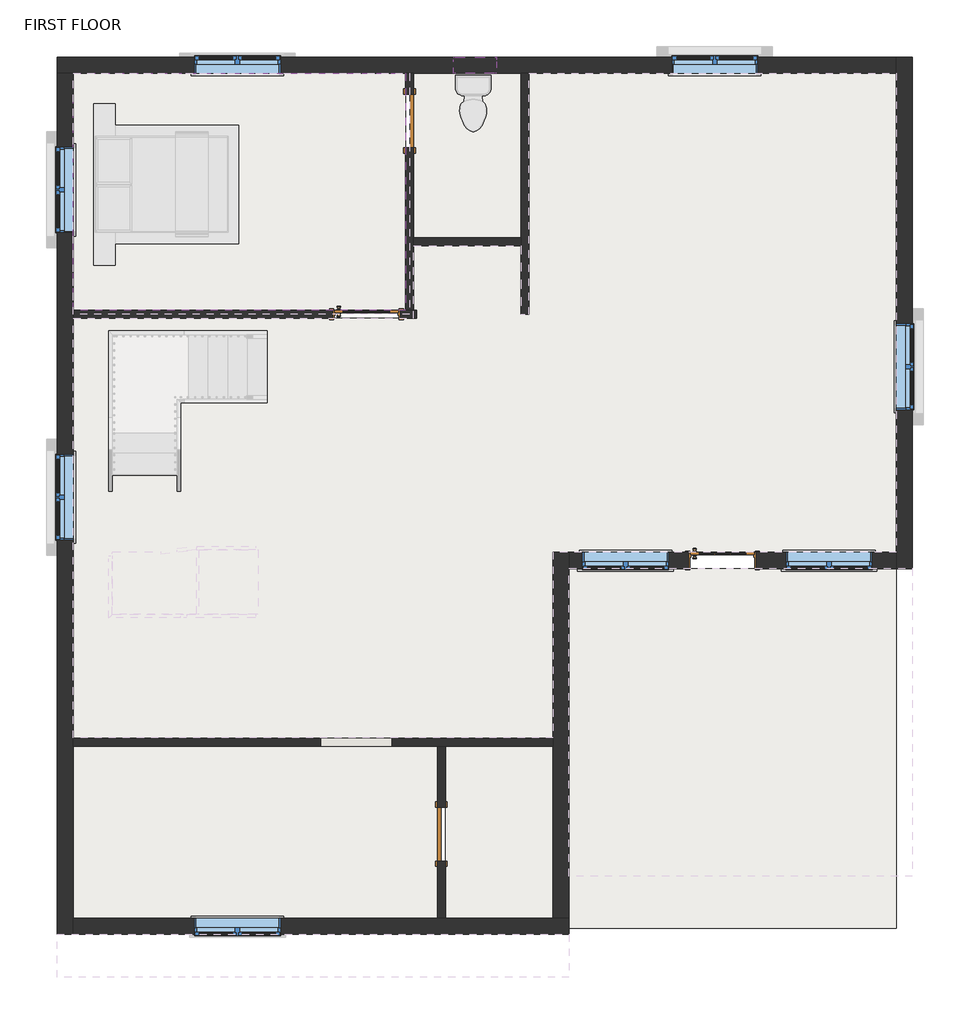
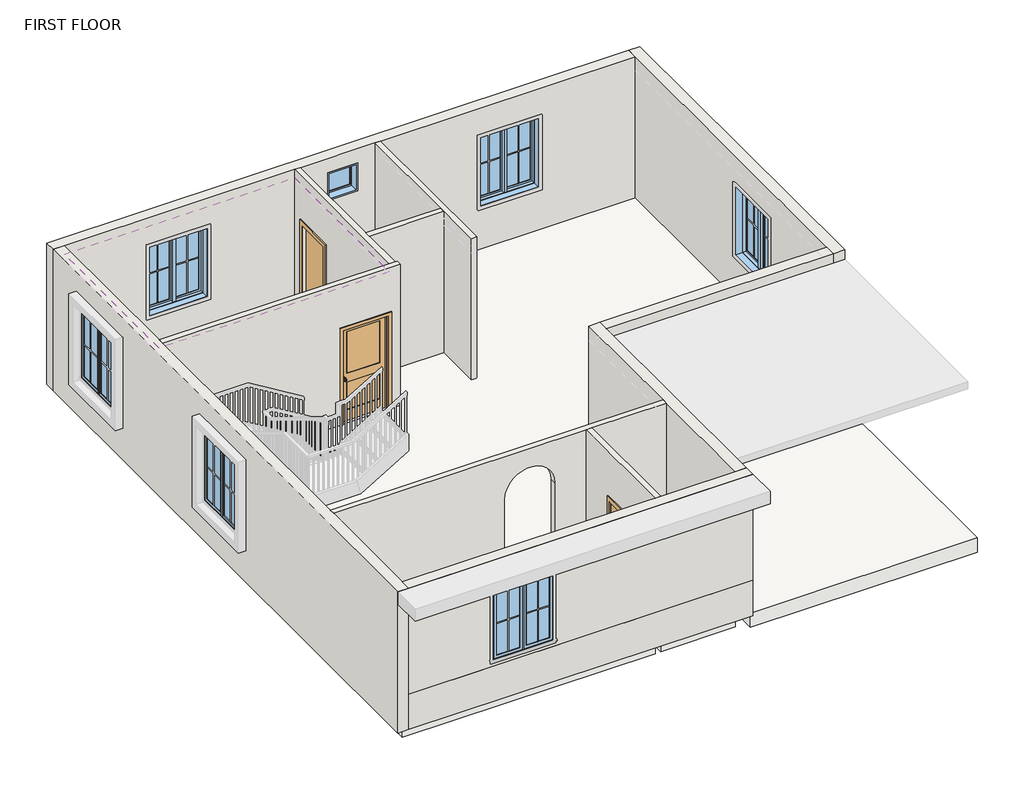
# One storey, part 1 of 4: 13 walls, 9 windows, 4 doors, 1 covering, 1 slab.
"""IFC4 building model written with IfcOpenShell, lengths in millimetres."""

from ifc_helpers import new_model, si_unit, frame, origin, place, context, project, spatial, polyline, circle_curve, outline, extrude, faceted_brep, transform, mapped, element, save
from ifc_brep_helpers import plane_surface, revolved_surface, advanced_brep
from components import door_29124af5, door_c89e1556, door_d8f5dbb5, window_80340324, window_8377141f

model = new_model("IFC4")

# Units and contexts
model_context = context("Model", 3, world=origin())
ifc_project = project(units=[si_unit("LENGTHUNIT", "METRE", prefix="MILLI")], contexts=[model_context])

# Site, building, storey
site = spatial("IfcSite", under=ifc_project)
building = spatial("IfcBuilding", under=site)
storey = spatial("IfcBuildingStorey", under=building, Name="FIRST FLOOR", Elevation=3352.8)

# Covering
placement = place(None, origin())
element("IfcCovering", 1, ObjectType="WHITE CEILING", at=placement, inside=storey, context=model_context, shape_type="SweptSolid", body=[
    extrude(outline(polyline([(-7115.7086008, 4742.0155883), (-7115.7086008, 1389.2155883), (-11821.0586008, 1389.2155883), (-11821.0586008, 4742.0155883), (-7115.7086008, 4742.0155883)])), frame((0.0, 0.0, 6223.0), z_axis=(0.0, 0.0, 1.0), x_axis=(1.0, 0.0, 0.0)), (0.0, 0.0, 1.0), 107.95),
])

# Doors
door_shape = door_29124af5(model_context)
element("IfcDoor", 2, ObjectType="Door-Interior-Single-2_Panel-Wood : 36\" x 80\"", at=placement, inside=storey, context=model_context, shape_type="MappedRepresentation", body=[
    mapped(door_shape, transform((-7668.1586008, 1335.2405883, 3352.8), x_axis=(1.0, 0.0, 0.0), y_axis=(0.0, 1.0, 0.0), z_axis=(0.0, 0.0, 1.0))),
])
door_2_shape = door_c89e1556(model_context)
element("IfcDoor", 3, ObjectType="Door-Interior-Single-Full Glass-Wood : 36\" x 84\"", at=placement, inside=storey, context=model_context, shape_type="MappedRepresentation", body=[
    mapped(door_2_shape, transform((-2626.2586008, -2150.9094117, 3352.8), x_axis=(1.0, 0.0, 0.0), y_axis=(0.0, 1.0, 0.0), z_axis=(0.0, 0.0, 1.0))),
])
door_3_shape = door_d8f5dbb5(model_context)
element("IfcDoor", 4, ObjectType="Single-Flush : 30\" x 80\"", at=placement, inside=storey, context=model_context, shape_type="MappedRepresentation", body=[
    mapped(door_3_shape, transform((-7058.5586008, 4068.9155883, 3352.8), x_axis=(0.0, -1.0, 0.0), y_axis=(1.0, 0.0, 0.0), z_axis=(0.0, 0.0, 1.0))),
])
element("IfcDoor", 5, ObjectType="Single-Flush : 30\" x 80\"", at=placement, inside=storey, context=model_context, shape_type="MappedRepresentation", body=[
    mapped(door_3_shape, transform((-6607.7086008, -6030.7594117, 3352.8), x_axis=(0.0, 1.0, 0.0), y_axis=(-1.0, 0.0, 0.0), z_axis=(0.0, 0.0, 1.0))),
])

# Slab
element("IfcSlab", 6, ObjectType="MARBLE FLOORING 1'", at=placement, inside=storey, context=model_context, shape_type="SweptSolid", body=[
    extrude(outline(polyline([(-7115.7086008, 4742.0155883), (-7115.7086008, 1389.2155883), (-11821.0586008, 1389.2155883), (-11821.0586008, 4742.0155883), (-7115.7086008, 4742.0155883)])), frame((0.0, 0.0, 3048.0), z_axis=(0.0, 0.0, 1.0), x_axis=(1.0, 0.0, 0.0)), (0.0, 0.0, 1.0), 304.8),
    extrude(outline(polyline([(-162.4586008, -2268.3844117), (-162.4586008, -7361.0844117), (-4797.9586008, -7361.0844117), (-4797.9586008, -2268.3844117), (-162.4586008, -2268.3844117)])), frame((0.0, 0.0, 3048.0), z_axis=(0.0, 0.0, 1.0), x_axis=(1.0, 0.0, 0.0)), (0.0, 0.0, 1.0), 304.8),
    extrude(outline(polyline([(-5477.4086008, 4742.0155883), (-5477.4086008, 2417.9155883), (-7001.4086008, 2417.9155883), (-7001.4086008, 4742.0155883), (-5477.4086008, 4742.0155883)])), frame((0.0, 0.0, 3048.0), z_axis=(0.0, 0.0, 1.0), x_axis=(1.0, 0.0, 0.0)), (0.0, 0.0, 1.0), 304.8),
    extrude(outline(polyline([(-6664.8586008, -4782.9844117), (-6664.8586008, -7221.3844117), (-11821.0586008, -7221.3844117), (-11821.0586008, -4782.9844117), (-6664.8586008, -4782.9844117)])), frame((0.0, 0.0, 3048.0), z_axis=(0.0, 0.0, 1.0), x_axis=(1.0, 0.0, 0.0)), (0.0, 0.0, 1.0), 304.8),
    extrude(outline(polyline([(-5026.5586008, -4782.9844117), (-5026.5586008, -7221.3844117), (-6550.5586008, -7221.3844117), (-6550.5586008, -4782.9844117), (-5026.5586008, -4782.9844117)])), frame((0.0, 0.0, 3048.0), z_axis=(0.0, 0.0, 1.0), x_axis=(1.0, 0.0, 0.0)), (0.0, 0.0, 1.0), 304.8),
    extrude(outline(polyline([(-11821.0586008, 1274.9155883), (-6956.9586008, 1274.9155883), (-6956.9586008, 1389.2155883), (-7001.4086008, 1389.2155883), (-7001.4086008, 2303.6155883), (-5477.4086008, 2303.6155883), (-5477.4086008, 1332.0655883), (-5363.1086008, 1332.0655883), (-5363.1086008, 4742.0155883), (-162.4586008, 4742.0155883), (-162.4586008, -2039.7844117), (-5026.5586008, -2039.7844117), (-5026.5586008, -4668.6844117), (-11821.0586008, -4668.6844117), (-11821.0586008, 1274.9155883)])), frame((0.0, 0.0, 3048.0), z_axis=(0.0, 0.0, 1.0), x_axis=(1.0, 0.0, 0.0)), (0.0, 0.0, 1.0), 304.8),
])

# Walls
element("IfcWall", 7, at=placement, inside=storey, context=model_context, shape_type="Brep", body=[
    faceted_brep([(-7115.7086008, 3687.9155883, 5384.8), (-7115.7086008, 3687.9155883, 3352.8), (-7115.7086008, 1389.2155883, 3352.8), (-7115.7086008, 1389.2155883, 6400.8), (-7115.7086008, 4742.0155883, 6400.8), (-7115.7086008, 4742.0155883, 3352.8), (-7115.7086008, 4449.9155883, 3352.8), (-7115.7086008, 4449.9155883, 5384.8), (-7001.4086008, 1389.2155883, 3352.8), (-7001.4086008, 2303.6155883, 3352.8), (-7001.4086008, 2417.9155883, 3352.8), (-7001.4086008, 3687.9155883, 3352.8), (-7001.4086008, 3687.9155883, 5384.8), (-7001.4086008, 4449.9155883, 5384.8), (-7001.4086008, 4449.9155883, 3352.8), (-7001.4086008, 4742.0155883, 3352.8), (-7001.4086008, 4742.0155883, 6400.8), (-7001.4086008, 2417.9155883, 6400.8), (-7001.4086008, 2303.6155883, 6400.8), (-7001.4086008, 1389.2155883, 6400.8)], [[[0, 1, 2, 3, 4, 5, 6, 7]], [[8, 9, 10, 11, 12, 13, 14, 15, 16, 17, 18, 19]], [[6, 5, 15, 14]], [[2, 1, 11, 10, 9, 8]], [[4, 3, 19, 18, 17, 16]], [[5, 4, 16, 15]], [[3, 2, 8, 19]], [[12, 11, 1, 0]], [[13, 12, 0, 7]], [[14, 13, 7, 6]]]),
])
element("IfcWall", 8, at=placement, inside=storey, context=model_context, shape_type="Brep", body=[
    faceted_brep([(-5477.4086008, 4742.0155883, 3352.8), (-5477.4086008, 2417.9155883, 3352.8), (-5477.4086008, 2303.6155883, 3352.8), (-5477.4086008, 1332.0655883, 3352.8), (-5477.4086008, 1332.0655883, 6400.8), (-5477.4086008, 2303.6155883, 6400.8), (-5477.4086008, 2417.9155883, 6400.8), (-5477.4086008, 4742.0155883, 6400.8), (-5363.1086008, 4742.0155883, 3352.8), (-5363.1086008, 4742.0155883, 6400.8), (-5363.1086008, 1332.0655883, 6400.8), (-5363.1086008, 1332.0655883, 3352.8)], [[[0, 1, 2, 3, 4, 5, 6, 7]], [[8, 9, 10, 11]], [[3, 2, 1, 0, 8, 11]], [[4, 3, 11, 10]], [[7, 6, 5, 4, 10, 9]], [[0, 7, 9, 8]]]),
])
element("IfcWall", 9, at=placement, inside=storey, context=model_context, shape_type="Brep", body=[
    faceted_brep([(-6956.9586008, 1274.9155883, 3352.8), (-6956.9586008, 1274.9155883, 6400.8), (-11821.0586008, 1274.9155883, 6400.8), (-11821.0586008, 1274.9155883, 3352.8), (-8150.7586008, 1274.9155883, 3352.8), (-8150.7586008, 1274.9155883, 5410.2), (-7185.5586008, 1274.9155883, 5410.2), (-7185.5586008, 1274.9155883, 3352.8), (-6956.9586008, 1389.2155883, 6400.8), (-6956.9586008, 1389.2155883, 3352.8), (-7001.4086008, 1389.2155883, 3352.8), (-7115.7086008, 1389.2155883, 3352.8), (-7185.5586008, 1389.2155883, 3352.8), (-7185.5586008, 1389.2155883, 5410.2), (-8150.7586008, 1389.2155883, 5410.2), (-8150.7586008, 1389.2155883, 3352.8), (-11821.0586008, 1389.2155883, 3352.8), (-11821.0586008, 1389.2155883, 6400.8), (-7115.7086008, 1389.2155883, 6400.8), (-7001.4086008, 1389.2155883, 6400.8)], [[[0, 1, 2, 3, 4, 5, 6, 7]], [[8, 9, 10, 11, 12, 13, 14, 15, 16, 17, 18, 19]], [[9, 0, 7, 12, 11, 10]], [[3, 16, 15, 4]], [[1, 0, 9, 8]], [[2, 1, 8, 19, 18, 17]], [[3, 2, 17, 16]], [[6, 13, 12, 7]], [[13, 6, 5, 14]], [[14, 5, 4, 15]]]),
])
element("IfcWall", 10, at=placement, inside=storey, context=model_context, shape_type="AdvancedBrep", body=[
    advanced_brep(
    [(-11821.0586008, -4782.9844117, 3352.8), (-6664.8586008, -4782.9844117, 3352.8), (-6550.5586008, -4782.9844117, 3352.8), (-5026.5586008, -4782.9844117, 3352.8), (-5026.5586008, -4782.9844117, 6400.8), (-6550.5586008, -4782.9844117, 6400.8), (-6664.8586008, -4782.9844117, 6400.8), (-11821.0586008, -4782.9844117, 6400.8), (-7306.1699369, -4782.9844117, 3400.7143117), (-8322.1699369, -4782.9844117, 3400.7143117), (-8322.1699369, -4782.9844117, 5483.5143117), (-7306.1699369, -4782.9844117, 5483.5143117), (-11821.0586008, -4668.6844117, 3352.8), (-11821.0586008, -4668.6844117, 6400.8), (-5026.5586008, -4668.6844117, 6400.8), (-5026.5586008, -4668.6844117, 3352.8), (-7306.1699369, -4668.6844117, 3400.7143117), (-7306.1699369, -4668.6844117, 5483.5143117), (-8322.1699369, -4668.6844117, 5483.5143117), (-8322.1699369, -4668.6844117, 3400.7143117)],
    [
        (0, 1),
        (1, 2),
        (2, 3),
        (3, 4),
        (4, 5),
        (5, 6),
        (6, 7),
        (7, 0),
        (8, 9),
        (9, 10),
        (10, 11, circle_curve(frame((-7814.1699369, -4782.9844117, 5483.5143117), z_axis=(0.0, 1.0, 0.0), x_axis=(-1.0, 0.0, 0.0)), 508.0)),
        (11, 8),
        (12, 13),
        (13, 14),
        (14, 15),
        (15, 12),
        (16, 17),
        (17, 18, circle_curve(frame((-7814.1699369, -4668.6844117, 5483.5143117), z_axis=(0.0, -1.0, 0.0), x_axis=(-1.0, 0.0, 0.0)), 508.0)),
        (18, 19),
        (19, 16),
        (7, 13),
        (12, 0),
        (3, 15),
        (14, 4),
        (8, 16),
        (19, 9),
        (18, 10),
        (17, 11),
    ],
    [
        plane_surface(frame((-11935.3586008, -4782.9844117, 3352.8), z_axis=(0.0, -1.0, 0.0), x_axis=(1.0, 0.0, 0.0))),
        plane_surface(frame((-11935.3586008, -4668.6844117, 3352.8), z_axis=(0.0, 1.0, 0.0), x_axis=(-1.0, 0.0, 0.0))),
        plane_surface(frame((-11821.0586008, 2722.7155883, 3352.8), z_axis=(-1.0, 0.0, 0.0), x_axis=(0.0, 1.0, 0.0))),
        plane_surface(frame((-5026.5586008, -7221.3844117, 3352.8), z_axis=(1.0, 0.0, 0.0), x_axis=(0.0, -1.0, 0.0))),
        plane_surface(frame((-11935.3586008, -4782.9844117, 3352.8), z_axis=(0.0, 0.0, -1.0), x_axis=(0.0, 1.0, 0.0))),
        plane_surface(frame((-4912.2586008, -4782.9844117, 6400.8), z_axis=(0.0, 0.0, 1.0), x_axis=(0.0, 1.0, 0.0))),
        plane_surface(frame((-7306.1699369, -4782.9844117, 3400.7143117), z_axis=(0.0, 0.0, 1.0), x_axis=(0.0, 1.0, 0.0))),
        plane_surface(frame((-8322.1699369, -4782.9844117, 3400.7143117), z_axis=(1.0, 0.0, 0.0), x_axis=(0.0, 1.0, 0.0))),
        revolved_surface(polyline([(-8322.1699369, -4668.6844117, 5483.5143117), (-8322.1699369, -4782.9844117, 5483.5143117)]), (-7814.1699369, -4725.8344117, 5483.5143117), (0.0, 1.0, 0.0)),
        plane_surface(frame((-7306.1699369, -4782.9844117, 5483.5143117), z_axis=(-1.0, 0.0, 0.0), x_axis=(0.0, 1.0, 0.0))),
    ],
    [
        (0, [[1, 2, 3, 4, 5, 6, 7, 8], [9, 10, 11, 12]]),
        (1, [[13, 14, 15, 16], [17, 18, 19, 20]]),
        (2, [[-8, 21, -13, 22]]),
        (3, [[-4, 23, -15, 24]]),
        (4, [[-3, -2, -1, -22, -16, -23]]),
        (5, [[-7, -6, -5, -24, -14, -21]]),
        (6, [[-9, 25, -20, 26]]),
        (7, [[-10, -26, -19, 27]]),
        (8, [[-11, -27, -18, 28]]),
        (9, [[-12, -28, -17, -25]]),
    ],
),
])
element("IfcWall", 11, at=placement, inside=storey, context=model_context, shape_type="SweptSolid", body=[
    extrude(outline(polyline([(-4782.9844117, 3352.8), (-5649.7594117, 3352.8), (-5649.7594117, 5384.8), (-6411.7594117, 5384.8), (-6411.7594117, 3352.8), (-7221.3844117, 3352.8), (-7221.3844117, 6400.8), (-4782.9844117, 6400.8), (-4782.9844117, 3352.8)])), frame((-6664.8586008, 0.0, 0.0), z_axis=(1.0, 0.0, 0.0), x_axis=(0.0, 1.0, 0.0)), (0.0, 0.0, 1.0), 114.3),
])
element("IfcWall", 12, at=placement, inside=storey, context=model_context, shape_type="SweptSolid", body=[
    extrude(outline(polyline([(-7001.4086008, 2417.9155883), (-5477.4086008, 2417.9155883), (-5477.4086008, 2303.6155883), (-7001.4086008, 2303.6155883), (-7001.4086008, 2417.9155883)])), frame((0.0, 0.0, 3352.8), z_axis=(0.0, 0.0, 1.0), x_axis=(1.0, 0.0, 0.0)), (0.0, 0.0, 1.0), 3048.0),
])
element("IfcWall", 13, ObjectType="OUTER WALL CREAM WHITE 9\"", at=placement, inside=storey, context=model_context, shape_type="Brep", body=[
    faceted_brep([(-12049.6586008, 4742.0155883, 3352.8), (-11821.0586008, 4742.0155883, 3352.8), (-7115.7086008, 4742.0155883, 3352.8), (-7001.4086008, 4742.0155883, 3352.8), (-5477.4086008, 4742.0155883, 3352.8), (-5363.1086008, 4742.0155883, 3352.8), (-162.4586008, 4742.0155883, 3352.8), (-162.4586008, 4742.0155883, 6400.8), (-5363.1086008, 4742.0155883, 6400.8), (-5477.4086008, 4742.0155883, 6400.8), (-7001.4086008, 4742.0155883, 6400.8), (-7115.7086008, 4742.0155883, 6400.8), (-11821.0586008, 4742.0155883, 6400.8), (-12049.6586008, 4742.0155883, 6400.8), (-8887.3586008, 4742.0155883, 5791.2), (-8887.3586008, 4742.0155883, 4267.2), (-10106.5586008, 4742.0155883, 4267.2), (-10106.5586008, 4742.0155883, 5791.2), (-2124.6086008, 4742.0155883, 5791.2), (-2124.6086008, 4742.0155883, 4267.2), (-3343.8086008, 4742.0155883, 4267.2), (-3343.8086008, 4742.0155883, 5791.2), (-5826.6586008, 4742.0155883, 6096.0), (-5826.6586008, 4742.0155883, 5486.4), (-6436.2586008, 4742.0155883, 5486.4), (-6436.2586008, 4742.0155883, 6096.0), (-12049.6586008, 4970.6155883, 3352.8), (-12049.6586008, 4970.6155883, 6400.8), (-162.4586008, 4970.6155883, 6400.8), (-162.4586008, 4970.6155883, 3352.8), (-8887.3586008, 4970.6155883, 5791.2), (-10106.5586008, 4970.6155883, 5791.2), (-10106.5586008, 4970.6155883, 4267.2), (-8887.3586008, 4970.6155883, 4267.2), (-2124.6086008, 4970.6155883, 5791.2), (-3343.8086008, 4970.6155883, 5791.2), (-3343.8086008, 4970.6155883, 4267.2), (-2124.6086008, 4970.6155883, 4267.2), (-5826.6586008, 4970.6155883, 6096.0), (-6436.2586008, 4970.6155883, 6096.0), (-6436.2586008, 4970.6155883, 5486.4), (-5826.6586008, 4970.6155883, 5486.4)], [[[0, 1, 2, 3, 4, 5, 6, 7, 8, 9, 10, 11, 12, 13], [14, 15, 16, 17], [18, 19, 20, 21], [22, 23, 24, 25]], [[26, 27, 28, 29], [30, 31, 32, 33], [34, 35, 36, 37], [38, 39, 40, 41]], [[6, 5, 4, 3, 2, 1, 0, 26, 29]], [[13, 12, 11, 10, 9, 8, 7, 28, 27]], [[0, 13, 27, 26]], [[7, 6, 29, 28]], [[15, 14, 30, 33]], [[16, 15, 33, 32]], [[17, 16, 32, 31]], [[14, 17, 31, 30]], [[19, 18, 34, 37]], [[20, 19, 37, 36]], [[21, 20, 36, 35]], [[18, 21, 35, 34]], [[23, 22, 38, 41]], [[24, 23, 41, 40]], [[25, 24, 40, 39]], [[22, 25, 39, 38]]]),
])
element("IfcWall", 14, ObjectType="OUTER WALL CREAM WHITE 9\"", at=placement, inside=storey, context=model_context, shape_type="Brep", body=[
    faceted_brep([(-11821.0586008, -7449.9844117, 6400.8), (-11821.0586008, -7449.9844117, 4114.8), (-11821.0586008, -7449.9844117, 3352.8), (-11821.0586008, -7221.3844117, 3352.8), (-11821.0586008, -4782.9844117, 3352.8), (-11821.0586008, -4668.6844117, 3352.8), (-11821.0586008, 1274.9155883, 3352.8), (-11821.0586008, 1389.2155883, 3352.8), (-11821.0586008, 4742.0155883, 3352.8), (-11821.0586008, 4742.0155883, 6400.8), (-11821.0586008, 1389.2155883, 6400.8), (-11821.0586008, 1274.9155883, 6400.8), (-11821.0586008, -4668.6844117, 6400.8), (-11821.0586008, -4782.9844117, 6400.8), (-11821.0586008, -7221.3844117, 6400.8), (-11821.0586008, 3703.7905883, 5791.2), (-11821.0586008, 3703.7905883, 4267.2), (-11821.0586008, 2484.5905883, 4267.2), (-11821.0586008, 2484.5905883, 5791.2), (-11821.0586008, -649.1344117, 5791.2), (-11821.0586008, -649.1344117, 4267.2), (-11821.0586008, -1868.3344117, 4267.2), (-11821.0586008, -1868.3344117, 5791.2), (-12049.6586008, -7449.9844117, 3352.8), (-12049.6586008, -7449.9844117, 6400.8), (-12049.6586008, 4742.0155883, 6400.8), (-12049.6586008, 4742.0155883, 3352.8), (-12049.6586008, 3703.7905883, 5791.2), (-12049.6586008, 2484.5905883, 5791.2), (-12049.6586008, 2484.5905883, 4267.2), (-12049.6586008, 3703.7905883, 4267.2), (-12049.6586008, -649.1344117, 5791.2), (-12049.6586008, -1868.3344117, 5791.2), (-12049.6586008, -1868.3344117, 4267.2), (-12049.6586008, -649.1344117, 4267.2)], [[[0, 1, 2, 3, 4, 5, 6, 7, 8, 9, 10, 11, 12, 13, 14], [15, 16, 17, 18], [19, 20, 21, 22]], [[23, 24, 25, 26], [27, 28, 29, 30], [31, 32, 33, 34]], [[8, 7, 6, 5, 4, 3, 2, 23, 26]], [[0, 14, 13, 12, 11, 10, 9, 25, 24]], [[9, 8, 26, 25]], [[16, 15, 27, 30]], [[17, 16, 30, 29]], [[18, 17, 29, 28]], [[15, 18, 28, 27]], [[20, 19, 31, 34]], [[21, 20, 34, 33]], [[22, 21, 33, 32]], [[19, 22, 32, 31]], [[0, 24, 23, 2, 1]]]),
])
element("IfcWall", 15, ObjectType="OUTER WALL CREAM WHITE 9\"", at=placement, inside=storey, context=model_context, shape_type="Brep", body=[
    faceted_brep([(-4797.9586008, -7221.3844117, 3352.8), (-5026.5586008, -7221.3844117, 3352.8), (-6550.5586008, -7221.3844117, 3352.8), (-6664.8586008, -7221.3844117, 3352.8), (-11821.0586008, -7221.3844117, 3352.8), (-11821.0586008, -7221.3844117, 4114.8), (-4797.9586008, -7221.3844117, 4114.8), (-4797.9586008, -7449.9844117, 3352.8), (-4797.9586008, -7449.9844117, 4114.8), (-11821.0586008, -7449.9844117, 4114.8), (-11821.0586008, -7449.9844117, 3352.8)], [[[0, 1, 2, 3, 4, 5, 6]], [[7, 8, 9, 10]], [[4, 3, 2, 1, 0, 7, 10]], [[6, 5, 9, 8]], [[5, 4, 10, 9]], [[0, 6, 8, 7]]]),
])
element("IfcWall", 16, ObjectType="OUTER WALL CREAM WHITE 9\"", at=placement, inside=storey, context=model_context, shape_type="Brep", body=[
    faceted_brep([(-162.4586008, 4970.6155883, 3352.8), (-162.4586008, 4742.0155883, 3352.8), (-162.4586008, -2039.7844117, 3352.8), (-162.4586008, -2268.3844117, 3352.8), (-162.4586008, -2268.3844117, 6400.8), (-162.4586008, -2039.7844117, 6400.8), (-162.4586008, 4742.0155883, 6400.8), (-162.4586008, 4970.6155883, 6400.8), (-162.4586008, -20.4844117, 5791.2), (-162.4586008, -20.4844117, 4267.2), (-162.4586008, 1198.7155883, 4267.2), (-162.4586008, 1198.7155883, 5791.2), (66.1413992, 4970.6155883, 3352.8), (66.1413992, 4970.6155883, 6400.8), (66.1413992, -2268.3844117, 6400.8), (66.1413992, -2268.3844117, 3352.8), (66.1413992, -20.4844117, 5791.2), (66.1413992, 1198.7155883, 5791.2), (66.1413992, 1198.7155883, 4267.2), (66.1413992, -20.4844117, 4267.2)], [[[0, 1, 2, 3, 4, 5, 6, 7], [8, 9, 10, 11]], [[12, 13, 14, 15], [16, 17, 18, 19]], [[3, 2, 1, 0, 12, 15]], [[4, 3, 15, 14]], [[7, 6, 5, 4, 14, 13]], [[0, 7, 13, 12]], [[9, 8, 16, 19]], [[10, 9, 19, 18]], [[11, 10, 18, 17]], [[8, 11, 17, 16]]]),
])
element("IfcWall", 17, ObjectType="OUTER WALL CREAM WHITE 9\"", at=placement, inside=storey, context=model_context, shape_type="Brep", body=[
    faceted_brep([(-4797.9586008, -7221.3844117, 6400.8), (-4797.9586008, -7221.3844117, 4114.8), (-4797.9586008, -7221.3844117, 3352.8), (-4797.9586008, -2268.3844117, 3352.8), (-4797.9586008, -2039.7844117, 3352.8), (-4797.9586008, -2039.7844117, 6400.8), (-4797.9586008, -2268.3844117, 6400.8), (-5026.5586008, -7221.3844117, 3352.8), (-5026.5586008, -7221.3844117, 6400.8), (-5026.5586008, -4782.9844117, 6400.8), (-5026.5586008, -4668.6844117, 6400.8), (-5026.5586008, -2039.7844117, 6400.8), (-5026.5586008, -2039.7844117, 3352.8), (-5026.5586008, -4668.6844117, 3352.8), (-5026.5586008, -4782.9844117, 3352.8)], [[[0, 1, 2, 3, 4, 5, 6]], [[7, 8, 9, 10, 11, 12, 13, 14]], [[4, 3, 2, 7, 14, 13, 12]], [[0, 6, 5, 11, 10, 9, 8]], [[5, 4, 12, 11]], [[0, 8, 7, 2, 1]]]),
])
element("IfcWall", 18, ObjectType="OUTER WALL CREAM WHITE 9\"", at=placement, inside=storey, context=model_context, shape_type="SweptSolid", body=[
    extrude(outline(polyline([(6400.8, -162.4586008), (6400.8, -4797.9586008), (3352.8, -4797.9586008), (3352.8, -3108.8586008), (5511.8, -3108.8586008), (5511.8, -2143.6586008), (3352.8, -2143.6586008), (3352.8, -162.4586008), (6400.8, -162.4586008)]), holes=[polyline([(5791.2, -1724.5586008), (5791.2, -505.3586008), (4267.2, -505.3586008), (4267.2, -1724.5586008), (5791.2, -1724.5586008)]), polyline([(5791.2, -4607.4586008), (5791.2, -3388.2586008), (4267.2, -3388.2586008), (4267.2, -4607.4586008), (5791.2, -4607.4586008)])]), frame((0.0, -2268.3844117, 0.0), z_axis=(0.0, 1.0, 0.0), x_axis=(0.0, 0.0, 1.0)), (0.0, 0.0, 1.0), 228.6),
])
element("IfcWall", 19, ObjectType="OUTER WALL CREAM WHITE 9\"", at=placement, inside=storey, context=model_context, shape_type="Brep", body=[
    faceted_brep([(-4797.9586008, -7221.3844117, 4114.8), (-11821.0586008, -7221.3844117, 4114.8), (-11821.0586008, -7221.3844117, 6400.8), (-5026.5586008, -7221.3844117, 6400.8), (-4797.9586008, -7221.3844117, 6400.8), (-10106.5586008, -7221.3844117, 5791.2), (-10106.5586008, -7221.3844117, 4267.2), (-8887.3586008, -7221.3844117, 4267.2), (-8887.3586008, -7221.3844117, 5791.2), (-4797.9586008, -7449.9844117, 4114.8), (-4797.9586008, -7449.9844117, 6400.8), (-11821.0586008, -7449.9844117, 6400.8), (-11821.0586008, -7449.9844117, 4114.8), (-10106.5586008, -7449.9844117, 5791.2), (-8887.3586008, -7449.9844117, 5791.2), (-8887.3586008, -7449.9844117, 4267.2), (-10106.5586008, -7449.9844117, 4267.2)], [[[0, 1, 2, 3, 4], [5, 6, 7, 8]], [[9, 10, 11, 12], [13, 14, 15, 16]], [[1, 0, 9, 12]], [[4, 3, 2, 11, 10]], [[5, 8, 14, 13]], [[8, 7, 15, 14]], [[7, 6, 16, 15]], [[6, 5, 13, 16]], [[0, 4, 10, 9]], [[2, 1, 12, 11]]]),
])

# Windows
window_shape = window_80340324(model_context)
element("IfcWindow", 20, ObjectType="Fixed : 24\" x 24\"", at=placement, inside=storey, context=model_context, shape_type="MappedRepresentation", body=[
    mapped(window_shape, transform((-6093.3586008, 4856.3155883, 4572.0), x_axis=(1.0, 0.0, 0.0), y_axis=(0.0, 1.0, 0.0), z_axis=(0.0, 0.0, 1.0))),
])
window_2_shape = window_8377141f(model_context)
element("IfcWindow", 21, ObjectType="Window-Casement-Double : BLACK MATERIAL 2\"", at=placement, inside=storey, context=model_context, shape_type="MappedRepresentation", body=[
    mapped(window_2_shape, transform((-1114.9586008, -2154.0844117, 3352.8), x_axis=(-1.0, 0.0, 0.0), y_axis=(0.0, -1.0, 0.0), z_axis=(0.0, 0.0, 1.0))),
])
element("IfcWindow", 22, ObjectType="Window-Casement-Double : BLACK MATERIAL 2\"", at=placement, inside=storey, context=model_context, shape_type="MappedRepresentation", body=[
    mapped(window_2_shape, transform((-3997.8586008, -2154.0844117, 3352.8), x_axis=(-1.0, 0.0, 0.0), y_axis=(0.0, -1.0, 0.0), z_axis=(0.0, 0.0, 1.0))),
])
element("IfcWindow", 23, ObjectType="Window-Casement-Double : BLACK MATERIAL 2\"", at=placement, inside=storey, context=model_context, shape_type="MappedRepresentation", body=[
    mapped(window_2_shape, transform((-9496.9586008, -7335.6844117, 3352.8), x_axis=(-1.0, 0.0, 0.0), y_axis=(0.0, -1.0, 0.0), z_axis=(0.0, 0.0, 1.0))),
])
element("IfcWindow", 24, ObjectType="Window-Casement-Double : BLACK MATERIAL 2\"", at=placement, inside=storey, context=model_context, shape_type="MappedRepresentation", body=[
    mapped(window_2_shape, transform((-48.1586008, 589.1155883, 3352.8), x_axis=(0.0, -1.0, 0.0), y_axis=(1.0, 0.0, 0.0), z_axis=(0.0, 0.0, 1.0))),
])
element("IfcWindow", 25, ObjectType="Window-Casement-Double : BLACK MATERIAL 2\"", at=placement, inside=storey, context=model_context, shape_type="MappedRepresentation", body=[
    mapped(window_2_shape, transform((-9496.9586008, 4856.3155883, 3352.8), x_axis=(1.0, 0.0, 0.0), y_axis=(0.0, 1.0, 0.0), z_axis=(0.0, 0.0, 1.0))),
])
element("IfcWindow", 26, ObjectType="Window-Casement-Double : BLACK MATERIAL 2\"", at=placement, inside=storey, context=model_context, shape_type="MappedRepresentation", body=[
    mapped(window_2_shape, transform((-11935.3586008, 3094.1905883, 3352.8), x_axis=(0.0, 1.0, 0.0), y_axis=(-1.0, 0.0, 0.0), z_axis=(0.0, 0.0, 1.0))),
])
element("IfcWindow", 27, ObjectType="Window-Casement-Double : BLACK MATERIAL 2\"", at=placement, inside=storey, context=model_context, shape_type="MappedRepresentation", body=[
    mapped(window_2_shape, transform((-11935.3586008, -1258.7344117, 3352.8), x_axis=(0.0, 1.0, 0.0), y_axis=(-1.0, 0.0, 0.0), z_axis=(0.0, 0.0, 1.0))),
])
element("IfcWindow", 28, ObjectType="Window-Casement-Double : BLACK MATERIAL 2\"", at=placement, inside=storey, context=model_context, shape_type="MappedRepresentation", body=[
    mapped(window_2_shape, transform((-2734.2086008, 4856.3155883, 3352.8), x_axis=(1.0, 0.0, 0.0), y_axis=(0.0, 1.0, 0.0), z_axis=(0.0, 0.0, 1.0))),
])

save(model, "model.ifc")

# Revit data of these elements
# Type "WHITE CEILING"
#   Assembly Code = "C3030220"
#   built-in parameter 1002203 = 1 (stored number, unit not read)
#   built-in parameter 1002202 = 1 (stored number, unit not read)
#   Layers, outside or top first: 0' - 3 5/8" "WHITE CEILING" (function 1); 0' - 0 5/8" "WHITE CEILING" (function 5)
# Type "Door-Interior-Single-2_Panel-Wood : 36\" x 80\""
#   Type Mark = "9"
#   Assembly Code = "C1020300"
#   Analytic Construction = "Wooden"
#   Top Rail = 0' - 4 11/16"
#   Thickness = 0' - 1 3/8"
#   Thermal Resistance (R) = 2.5876 (h·ft²·°F)/BTU
#   Swing Angle [instance default] = 90.00°
#   Stiles = 0' - 4 3/4"
#   Rough Width = 3' - 2"
#   Rough Height = 6' - 9"
#   Lock Rail = 0' - 7 1/2"
#   Height = 6' - 8"
#   Width = 3' - 0"
#   Heat Transfer Coefficient (U) = 0.3865 BTU/(h·ft²·°F)
#   Bottom Rail = 0' - 9 1/8"
#   Trim Material = Cherry
#   Panel Material = Cherry
#   Frame Material = Cherry
#   Door Handle Material = Aluminum
#   Visual Light Transmittance = 0
#   Solar Heat Gain Coefficient = 0
#   Wall Closure = (empty or 0)
#   Function = (empty or 0)
# Type "Door-Interior-Single-Full Glass-Wood : 36\" x 84\""
#   Type Mark = "8"
#   Assembly Code = "C1020300"
#   Analytic Construction = "Wood frame with single clear glass"
#   Top Rail = 0' - 4 11/16"
#   Thickness = 0' - 1 3/8"
#   Thermal Resistance (R) = 1.0102 (h·ft²·°F)/BTU
#   Swing Angle [instance default] = 90.00°
#   Stiles = 0' - 4 3/4"
#   Rough Width = 3' - 2"
#   Rough Height = 7' - 1"
#   Height = 7' - 0"
#   Width = 3' - 0"
#   Heat Transfer Coefficient (U) = 0.9900 BTU/(h·ft²·°F)
#   Bottom Rail = 0' - 9 1/8"
#   Show Grill [instance default] = yes
#   Trim Material = Cherry
#   Panel Material = Cherry
#   Frame Material = Cherry
#   Door Handle Material = Aluminum
#   Visual Light Transmittance = 0
#   Solar Heat Gain Coefficient = 0
#   Wall Closure = (empty or 0)
#   Function = (empty or 0)
# Type "Single-Flush : 30\" x 80\""
#   Type Mark = "5"
#   Construction Type Id = "MDOOR"
#   Assembly Code = "C1020"
#   Analytic Construction = "Metal"
#   Thickness = 0' - 2"
#   Heat Transfer Coefficient (U) = 0.651978 BTU/(h·ft²·°F)
#   Height = 6' - 8"
#   Trim Projection Ext = 0' - 1"
#   Trim Projection Int = 0' - 1"
#   Trim Width = 0' - 3"
#   Width = 2' - 6"
#   Define Thermal Properties by = 1
#   Define Thermal Properties by = 1
#   Door Material = Door - Panel
#   Frame Material = Door - Frame
#   Visual Light Transmittance = 0
#   Solar Heat Gain Coefficient = 0
#   Function = (empty or 0)
#   Wall Closure = (empty or 0)
# Type "MARBLE FLOORING 1'"
#   Assembly Code = "B1010"
#   Function = 0
#   Layers, outside or top first: 1' - 0" "MARBLE MATERIAL" (function 1)
# Type
#   Assembly Code = "B2010"
#   Layers, outside or top first: 0' - 4 1/2" "OFF WHITE COLOUR" (function 1)
# Type "OUTER WALL CREAM WHITE 9\""
#   Assembly Code = "B2010"
#   Layers, outside or top first: 0' - 9" "OFF WHITE COLOUR" (function 1)
# Type "Fixed : 24\" x 24\""
#   Type Mark = "3"
#   Construction Type Id = "GSP4R"
#   Assembly Code = "B2020100"
#   Analytic Construction = "1/8 in Pilkington single glazing"
#   Visual Light Transmittance = 0.9
#   Solar Heat Gain Coefficient = 0.78
#   Heat Transfer Coefficient (U) = 0.6496 BTU/(h·ft²·°F)
#   Height = 2' - 0"
#   Default Sill Height = 3' - 0"
#   Width = 2' - 0"
#   Window Inset = 0' - 0 3/4"
#   Define Thermal Properties by = 1
#   Define Thermal Properties by = 1
#   Glass Pane Material = Glass
#   Sash Material = Sash
#   Wall Closure = (empty or 0)
# Type "Window-Casement-Double : BLACK MATERIAL 2\""
#   Type Mark = "18"
#   Fire Rating = "0.5h"
#   Assembly Code = "B2020100"
#   Analytic Construction = "Double glazing - domestic"
#   Frame Extension [instance default] = 0' - 0 1/4"
#   Window Inset [instance default] = 0' - 0"
#   Wall Thickness [instance default] = 0' - 6"
#   Interior Wall Closure [instance default] = 0' - 2 1/4"
#   Half Width = 2' - 0"
#   Visual Light Transmittance = 0.81
#   Thermal Resistance (R) = 1.8146 (h·ft²·°F)/BTU
#   Solar Heat Gain Coefficient = 0.76
#   Rough Width = 4' - 0 1/2"
#   Rough Height = 5' - 0 1/2"
#   Height = 5' - 0"
#   Heat Transfer Coefficient (U) = 0.5511 BTU/(h·ft²·°F)
#   Exterior Wall Closure [instance default] = 0' - 1 1/4"
#   Extension Jamb [instance default] = 0' - 2 1/4"
#   Default Sill Height = 3' - 0"
#   Width = 4' - 0"
#   Muntin Visibility = yes
#   Interior Trim Visibility [instance default] = yes
#   Exterior Trim Visibility [instance default] = yes
#   Extension Jamb Visibility [instance default] = yes
#   Interior Trim Material = Wood - Stained
#   Muntin Pattern = Muntin Pattern_2x2 : Muntin Pattern_2x2
#   Interior Trim = Trim-Window-Interior-Flat : Picture Frame
#   Interior Frame Material = Wood - Stained
#   Glass Panel Material = Glass
#   Exterior Trim Material = BLACK MATERIAL
#   Exterior Trim = Trim-Window-Exterior-Flat : with Sill
#   Exterior Frame Material = BLACK MATERIAL
#   Wall Closure = (empty or 0)
# Element 1 (IfcCovering, "WHITE CEILING")
#   Height Offset From Level = 9' - 5"
#   Phase Created = New Construction
#   Materials on its faces: "WHITE CEILING"
# Element 2 (IfcDoor, "Door-Interior-Single-2_Panel-Wood : 36\" x 80\"")
#   Swing Angle = 90.00°
#   Phase Created = New Construction
#   Materials on its faces: "Cherry", "Aluminum"
# Element 3 (IfcDoor, "Door-Interior-Single-Full Glass-Wood : 36\" x 84\"")
#   Swing Angle = 90.00°
#   Show Grill = yes
#   Phase Created = New Construction
#   Materials on its faces: "Cherry", "Aluminum", "Glass"
# Elements 4, 5 (IfcDoor, "Single-Flush : 30\" x 80\"")
#   Phase Created = New Construction
#   Materials on its faces: "Door - Frame", "Door - Panel"
# Element 6 (IfcSlab, "MARBLE FLOORING 1'")
#   Height Offset From Level = 0' - 0"
#   Phase Created = New Construction
#   Materials on its faces: "MARBLE MATERIAL"
# Elements 7, 8, 9, 10, 11, 12 (IfcWall)
#   Top Offset = 0' - 0"
#   Base Offset = 0' - 0"
#   wall height = 10' - 0"
#   Phase Created = New Construction
#   Base Constraint = FIRST FLOOR
#   Top Constraint = top of roof
#   Materials on its faces: "OFF WHITE COLOUR"
# Elements 13, 14, 16, 17, 18 (IfcWall, "OUTER WALL CREAM WHITE 9\"")
#   Top Offset = 0' - 0"
#   Base Offset = 0' - 0"
#   wall height = 10' - 0"
#   Phase Created = New Construction
#   Base Constraint = FIRST FLOOR
#   Top Constraint = top of roof
#   Materials on its faces: "OFF WHITE COLOUR"
# Element 15 (IfcWall, "OUTER WALL CREAM WHITE 9\"")
#   Top Offset = 0' - 0"
#   Base Offset = 0' - 0"
#   Unconnected Height = 2' - 6"
#   wall height = 2' - 6"
#   Phase Created = New Construction
#   Base Constraint = FIRST FLOOR
#   Materials on its faces: "OFF WHITE COLOUR"
# Element 19 (IfcWall, "OUTER WALL CREAM WHITE 9\"")
#   built-in parameter 1001111 = 2' - 6"
#   Top Offset = 0' - 0"
#   Base Offset = 2' - 6"
#   Unconnected Height = 7' - 6"
#   wall height = 7' - 6"
#   Phase Created = New Construction
#   Base Constraint = FIRST FLOOR
#   Top Constraint = top of roof
#   Materials on its faces: "OFF WHITE COLOUR"
# Element 20 (IfcWindow, "Fixed : 24\" x 24\"")
#   Mark = "18"
#   Phase Created = New Construction
#   Materials on its faces: "Sash", "Glass"
# Element 21 (IfcWindow, "Window-Casement-Double : BLACK MATERIAL 2\"")
#   Mark = "10"
#   Window Inset = 0' - 0"
#   Interior Wall Closure = 0' - 2 1/4"
#   Frame Extension = 0' - 0 1/4"
#   Exterior Wall Closure = 0' - 1 1/4"
#   Interior Trim Visibility = yes
#   Exterior Trim Visibility = yes
#   Phase Created = New Construction
#   Materials on its faces: "Wood - Stained", "Glass", "BLACK MATERIAL"
# Element 22 (IfcWindow, "Window-Casement-Double : BLACK MATERIAL 2\"")
#   Mark = "11"
#   Window Inset = 0' - 0"
#   Interior Wall Closure = 0' - 2 1/4"
#   Frame Extension = 0' - 0 1/4"
#   Exterior Wall Closure = 0' - 1 1/4"
#   Interior Trim Visibility = yes
#   Exterior Trim Visibility = yes
#   Phase Created = New Construction
#   Materials on its faces: "Wood - Stained", "Glass", "BLACK MATERIAL"
# Element 23 (IfcWindow, "Window-Casement-Double : BLACK MATERIAL 2\"")
#   Mark = "12"
#   Window Inset = 0' - 0"
#   Interior Wall Closure = 0' - 2 1/4"
#   Frame Extension = 0' - 0 1/4"
#   Exterior Wall Closure = 0' - 1 1/4"
#   Interior Trim Visibility = yes
#   Exterior Trim Visibility = yes
#   Phase Created = New Construction
#   Materials on its faces: "Wood - Stained", "Glass", "BLACK MATERIAL"
# Element 24 (IfcWindow, "Window-Casement-Double : BLACK MATERIAL 2\"")
#   Mark = "13"
#   Window Inset = 0' - 0"
#   Interior Wall Closure = 0' - 2 1/4"
#   Frame Extension = 0' - 0 1/4"
#   Exterior Wall Closure = 0' - 1 1/4"
#   Interior Trim Visibility = yes
#   Exterior Trim Visibility = yes
#   Phase Created = New Construction
#   Materials on its faces: "Wood - Stained", "Glass", "BLACK MATERIAL"
# Element 25 (IfcWindow, "Window-Casement-Double : BLACK MATERIAL 2\"")
#   Mark = "14"
#   Window Inset = 0' - 0"
#   Interior Wall Closure = 0' - 2 1/4"
#   Frame Extension = 0' - 0 1/4"
#   Exterior Wall Closure = 0' - 1 1/4"
#   Interior Trim Visibility = yes
#   Exterior Trim Visibility = yes
#   Phase Created = New Construction
#   Materials on its faces: "Wood - Stained", "Glass", "BLACK MATERIAL"
# Element 26 (IfcWindow, "Window-Casement-Double : BLACK MATERIAL 2\"")
#   Mark = "15"
#   Window Inset = 0' - 0"
#   Interior Wall Closure = 0' - 2 1/4"
#   Frame Extension = 0' - 0 1/4"
#   Exterior Wall Closure = 0' - 1 1/4"
#   Interior Trim Visibility = yes
#   Exterior Trim Visibility = yes
#   Phase Created = New Construction
#   Materials on its faces: "Wood - Stained", "Glass", "BLACK MATERIAL"
# Element 27 (IfcWindow, "Window-Casement-Double : BLACK MATERIAL 2\"")
#   Mark = "16"
#   Window Inset = 0' - 0"
#   Interior Wall Closure = 0' - 2 1/4"
#   Frame Extension = 0' - 0 1/4"
#   Exterior Wall Closure = 0' - 1 1/4"
#   Interior Trim Visibility = yes
#   Exterior Trim Visibility = yes
#   Phase Created = New Construction
#   Materials on its faces: "Wood - Stained", "Glass", "BLACK MATERIAL"
# Element 28 (IfcWindow, "Window-Casement-Double : BLACK MATERIAL 2\"")
#   Mark = "17"
#   Window Inset = 0' - 0"
#   Interior Wall Closure = 0' - 2 1/4"
#   Frame Extension = 0' - 0 1/4"
#   Exterior Wall Closure = 0' - 1 1/4"
#   Interior Trim Visibility = yes
#   Exterior Trim Visibility = yes
#   Phase Created = New Construction
#   Materials on its faces: "Wood - Stained", "Glass", "BLACK MATERIAL"
# Materials
#   "WHITE CEILING": class "Generic", colour RGB 120 120 120, transparency 0, Cost = 0
#   "Cherry": class "Wood", colour RGB 226 177 128, transparency 0, Description = "Prunus Serotina", Cost = 0
#   "Aluminum": class "Metal", colour RGB 247 247 247, transparency 0, Description = "Aluminum 6061", Cost = 0
#   "Door - Panel": class "Wood", colour RGB 210 159 95, transparency 0, Cost = 0
#   "Door - Frame": colour RGB 118 70 51, transparency 0, Cost = 0
#   "MARBLE MATERIAL": class "Generic", colour RGB 120 120 120, transparency 0, Cost = 0
#   "OFF WHITE COLOUR": class "Generic", colour RGB 120 120 120, transparency 0, Cost = 0
#   "Glass": class "Glass", colour RGB 0 128 192, transparency 0.75, Description = "Soda Lime Glass", Cost = 0
#   "Sash": class "Wood", colour RGB 224 178 126, transparency 0, Cost = 0
#   "Wood - Stained": class "Wood", colour RGB 224 178 126, transparency 0, Cost = 0
#   "BLACK MATERIAL": class "Generic", colour RGB 120 120 120, transparency 0, Cost = 0
